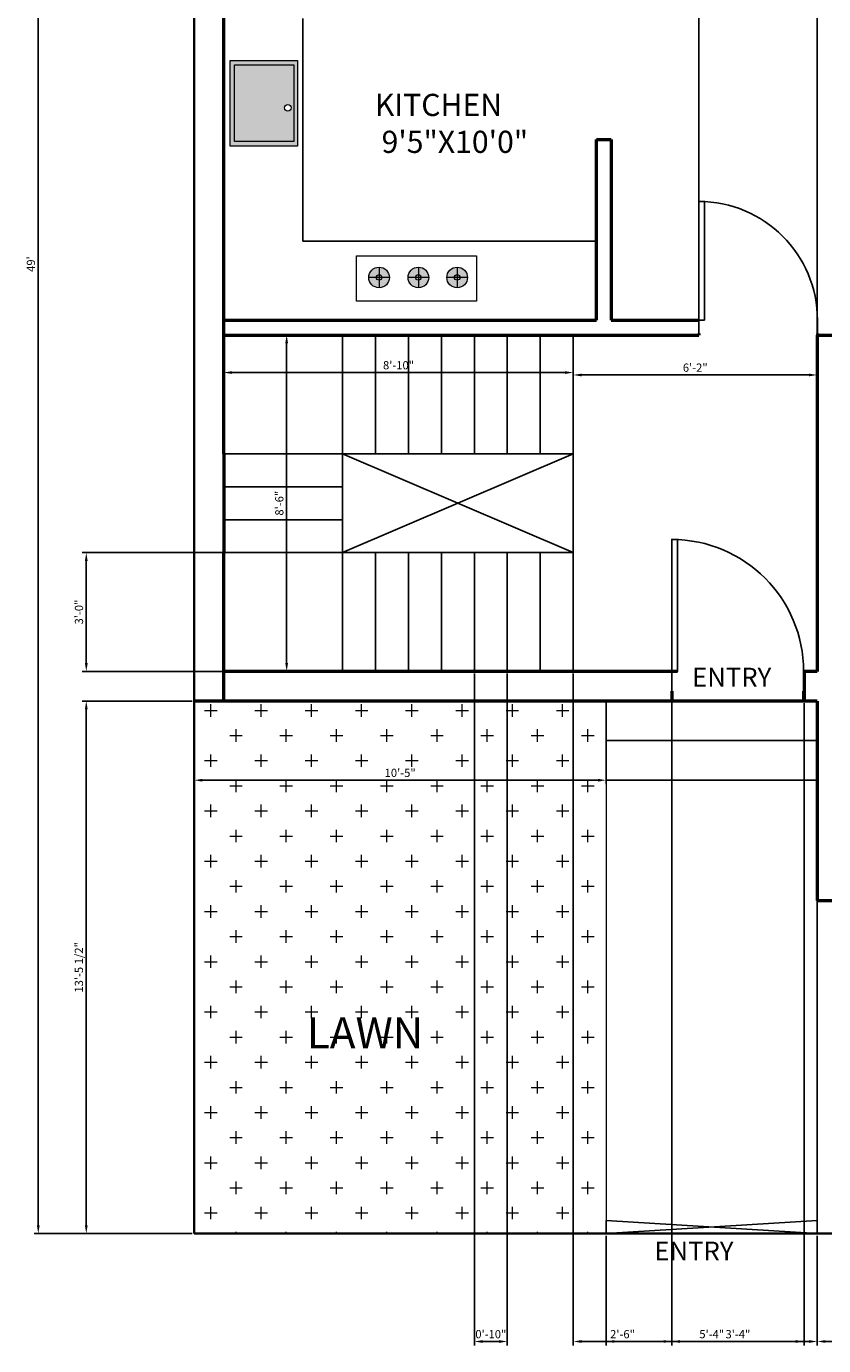
# Model space of a CAD drawing. Units: inches. Extents: x 1455 to 2044, y 1728 to 2439.
# Tile 1 of 4: x 1455 to 1697, y 1728 to 2128. Entities that reach past the tile are written whole.
import ezdxf

# ---------------------------------------------------------------- set-up
doc = ezdxf.new("R2010")
doc.units = ezdxf.units.IN
for name, color, linetype, lineweight in [('A-ANNO-DIMS', 2, 'Continuous', 18), ('A-ANNO-TEXT', 7, 'Continuous', 18), ('A-AREA-IDEN', 7, 'Continuous', 25), ('A-DOOR', 4, 'Continuous', 25), ('A-EQPM', 8, 'Continuous', 18), ('A-EQPM-PATT', 252, 'Continuous', 13), ('A-FLOR', 7, 'Continuous', 25), ('A-FLOR-CASE', 8, 'Continuous', 25), ('A-FLOR-FIXT', 9, 'Continuous', 18), ('A-FLOR-FIXT-PATT', 252, 'Continuous', 13), ('A-FLOR-STRS', 7, 'Continuous', 25), ('A-WALL', 7, 'Continuous', 50), ('C-PROP', 7, 'Continuous', 35), ('C-SITE-GATE', 1, 'Continuous', 25), ('L-PLNT', 3, 'Continuous', 18), ('L-PLNT-PATT', 3, 'Continuous', 13)]:
    doc.layers.add(name, color=color, linetype=linetype, lineweight=lineweight)
doc.styles.get("Standard").update_dxf_attribs({"font": 'arial.ttf'})
doc.dimstyles.new('ISO-25', dxfattribs={"dimtxt": 2.5, "dimasz": 2.5, "dimexe": 1.25, "dimexo": 0.625, "dimtad": 1, "dimlunit": 3, "dimtxsty": 'Standard', "dimcen": 2.5, "dimadec": 0, "dimazin": 0, "dimtfac": 1, "dimtmove": 0, "dimatfit": 3, "dimfxl": 1, "dimarcsym": 0})

# ---------------------------------------------------------------- blocks, each defined once
blk = doc.blocks.new('*D8')
at = {"layer": 'A-ANNO-DIMS', "color": 0, "lineweight": -2, "transparency": 16777216}
for p, q in [((1515.2, 2034.08), (1534.9, 2034.08)), ((1533.65, 2031.58), (1533.65, 1934.58)), ((1515.2, 1932.08), (1534.9, 1932.08))]:
    blk.add_line(p, q, dxfattribs=at)
at = {"layer": 'A-ANNO-DIMS', "color": 0, "transparency": 16777216}
for points in [[(1533.24, 2031.58), (1534.07, 2031.58), (1533.65, 2034.08)], [(1533.24, 1934.58), (1534.07, 1934.58), (1533.65, 1932.08)]]:
    blk.add_solid(points, dxfattribs=at)
at = {"layer": 'Defpoints', "color": 0, "transparency": 16777216}
for p in [(1514.58, 2034.08), (1514.58, 1932.08), (1533.65, 1932.08)]:
    blk.add_point(p, dxfattribs=at)
at = {"layer": 'A-ANNO-DIMS', "color": 0, "transparency": 16777216, "insert": (1531.75, 1983.08), "char_height": 2.5, "attachment_point": 5, "rotation": 90}
blk.add_mtext('8\'-6"', dxfattribs=at)
blk = doc.blocks.new('*D9')
at = {"layer": 'A-ANNO-DIMS', "color": 0, "lineweight": -2, "transparency": 16777216}
for p, q in [((1514.58, 2033.45), (1514.58, 2021.44)), ((1620.58, 2033.45), (1620.58, 2021.44)), ((1517.08, 2022.69), (1618.08, 2022.69))]:
    blk.add_line(p, q, dxfattribs=at)
at = {"layer": 'A-ANNO-DIMS', "color": 0, "transparency": 16777216}
for points in [[(1517.08, 2023.11), (1517.08, 2022.28), (1514.58, 2022.69)], [(1618.08, 2023.11), (1618.08, 2022.28), (1620.58, 2022.69)]]:
    blk.add_solid(points, dxfattribs=at)
at = {"layer": 'Defpoints', "color": 0, "transparency": 16777216}
for p in [(1514.58, 2034.08), (1620.58, 2034.08), (1620.58, 2022.69)]:
    blk.add_point(p, dxfattribs=at)
at = {"layer": 'A-ANNO-DIMS', "color": 0, "transparency": 16777216, "insert": (1567.58, 2024.59), "char_height": 2.5, "attachment_point": 5}
blk.add_mtext('8\'-10"', dxfattribs=at)
blk = doc.blocks.new('*D10')
at = {"layer": 'A-ANNO-DIMS', "color": 0, "lineweight": -2, "transparency": 16777216}
for p, q in [((1620.58, 2033.45), (1620.58, 2020.71)), ((1694.58, 2033.45), (1694.58, 2020.71)), ((1623.08, 2021.96), (1692.08, 2021.96))]:
    blk.add_line(p, q, dxfattribs=at)
at = {"layer": 'A-ANNO-DIMS', "color": 0, "transparency": 16777216}
for points in [[(1623.08, 2022.37), (1623.08, 2021.54), (1620.58, 2021.96)], [(1692.08, 2022.37), (1692.08, 2021.54), (1694.58, 2021.96)]]:
    blk.add_solid(points, dxfattribs=at)
at = {"layer": 'Defpoints', "color": 0, "transparency": 16777216}
for p in [(1620.58, 2034.08), (1694.58, 2034.08), (1694.58, 2021.96)]:
    blk.add_point(p, dxfattribs=at)
at = {"layer": 'A-ANNO-DIMS', "color": 0, "transparency": 16777216, "insert": (1657.58, 2023.86), "char_height": 2.5, "attachment_point": 5}
blk.add_mtext('6\'-2"', dxfattribs=at)
blk = doc.blocks.new('*U11')
for p, q in [((0, 0), (0, -6)), ((40, 0), (40, -6))]:
    blk.add_line(p, q)
blk.add_lwpolyline([(0, 0), (0, 40), (1.75, 40), (1.75, 0)], close=True)
blk.add_arc((0, 0), 40, 0, 90)
blk = doc.blocks.new('*U12')
for p, q in [((0, 0), (0, -4)), ((36, 0), (36, -4))]:
    blk.add_line(p, q)
blk.add_lwpolyline([(0, 0), (0, 36), (1.75, 36), (1.75, 0)], close=True)
blk.add_arc((0, 0), 36, 0, 90)
blk = doc.blocks.new('*D15')
at = {"layer": 'A-ANNO-DIMS', "color": 0, "lineweight": -2, "transparency": 16777216}
for p, q in [((1505.58, 1922.45), (1505.58, 1897.83)), ((1630.58, 1922.45), (1630.58, 1897.83)), ((1508.08, 1899.08), (1628.08, 1899.08))]:
    blk.add_line(p, q, dxfattribs=at)
at = {"layer": 'A-ANNO-DIMS', "color": 0, "transparency": 16777216}
for points in [[(1508.08, 1899.5), (1508.08, 1898.66), (1505.58, 1899.08)], [(1628.08, 1899.5), (1628.08, 1898.66), (1630.58, 1899.08)]]:
    blk.add_solid(points, dxfattribs=at)
at = {"layer": 'Defpoints', "color": 0, "transparency": 16777216}
for p in [(1505.58, 1923.08), (1630.58, 1923.08), (1630.58, 1899.08)]:
    blk.add_point(p, dxfattribs=at)
at = {"layer": 'A-ANNO-DIMS', "color": 0, "transparency": 16777216, "insert": (1568.08, 1900.98), "char_height": 2.5, "attachment_point": 5}
blk.add_mtext('10\'-5"', dxfattribs=at)
blk = doc.blocks.new('*D16')
at = {"layer": 'A-ANNO-DIMS', "color": 0, "lineweight": -2, "transparency": 16777216}
for p, q in [((1504.95, 2349.58), (1457.06, 2349.58)), ((1458.31, 2347.08), (1458.31, 1764.08)), ((1504.95, 1761.58), (1457.06, 1761.58))]:
    blk.add_line(p, q, dxfattribs=at)
at = {"layer": 'A-ANNO-DIMS', "color": 0, "transparency": 16777216}
for points in [[(1457.9, 2347.08), (1458.73, 2347.08), (1458.31, 2349.58)], [(1457.9, 1764.08), (1458.73, 1764.08), (1458.31, 1761.58)]]:
    blk.add_solid(points, dxfattribs=at)
at = {"layer": 'Defpoints', "color": 0, "transparency": 16777216}
for p in [(1505.58, 2349.58), (1458.31, 1761.58), (1505.58, 1761.58)]:
    blk.add_point(p, dxfattribs=at)
at = {"layer": 'A-ANNO-DIMS', "color": 0, "transparency": 16777216, "insert": (1456.41, 2055.58), "char_height": 2.5, "attachment_point": 5, "rotation": 90}
blk.add_mtext("49'", dxfattribs=at)
blk = doc.blocks.new('*D28')
at = {"layer": 'A-ANNO-DIMS', "color": 0, "lineweight": -2, "transparency": 16777216}
for p, q in [((1694.58, 1760.95), (1694.58, 1727.63)), ((1856.58, 1760.95), (1856.58, 1727.63)), ((1697.08, 1728.88), (1854.08, 1728.88))]:
    blk.add_line(p, q, dxfattribs=at)
at = {"layer": 'A-ANNO-DIMS', "color": 0, "transparency": 16777216}
for points in [[(1697.08, 1729.3), (1697.08, 1728.46), (1694.58, 1728.88)], [(1854.08, 1729.3), (1854.08, 1728.46), (1856.58, 1728.88)]]:
    blk.add_solid(points, dxfattribs=at)
at = {"layer": 'Defpoints', "color": 0, "transparency": 16777216}
for p in [(1694.58, 1761.58), (1856.58, 1761.58), (1856.58, 1728.88)]:
    blk.add_point(p, dxfattribs=at)
at = {"layer": 'A-ANNO-DIMS', "color": 0, "transparency": 16777216, "insert": (1775.58, 1730.78), "char_height": 2.5, "attachment_point": 5}
blk.add_mtext('13\'-6"', dxfattribs=at)
blk = doc.blocks.new('*D29')
at = {"layer": 'A-ANNO-DIMS', "color": 0, "lineweight": -2, "transparency": 16777216}
for p, q in [((1630.58, 1760.95), (1630.58, 1727.63)), ((1694.58, 1760.95), (1694.58, 1727.63)), ((1633.08, 1728.88), (1692.08, 1728.88))]:
    blk.add_line(p, q, dxfattribs=at)
at = {"layer": 'A-ANNO-DIMS', "color": 0, "transparency": 16777216}
for points in [[(1633.08, 1729.3), (1633.08, 1728.46), (1630.58, 1728.88)], [(1692.08, 1729.3), (1692.08, 1728.46), (1694.58, 1728.88)]]:
    blk.add_solid(points, dxfattribs=at)
at = {"layer": 'Defpoints', "color": 0, "transparency": 16777216}
for p in [(1630.58, 1761.58), (1694.58, 1761.58), (1694.58, 1728.88)]:
    blk.add_point(p, dxfattribs=at)
at = {"layer": 'A-ANNO-DIMS', "color": 0, "transparency": 16777216, "insert": (1662.58, 1730.78), "char_height": 2.5, "attachment_point": 5}
blk.add_mtext('5\'-4"', dxfattribs=at)
blk = doc.blocks.new('*D30')
at = {"layer": 'A-ANNO-DIMS', "color": 0, "lineweight": -2, "transparency": 16777216}
for p, q in [((1504.95, 1923.08), (1471.63, 1923.08)), ((1472.88, 1920.58), (1472.88, 1764.08)), ((1504.95, 1761.58), (1471.63, 1761.58))]:
    blk.add_line(p, q, dxfattribs=at)
at = {"layer": 'A-ANNO-DIMS', "color": 0, "transparency": 16777216}
for points in [[(1472.46, 1920.58), (1473.3, 1920.58), (1472.88, 1923.08)], [(1472.46, 1764.08), (1473.3, 1764.08), (1472.88, 1761.58)]]:
    blk.add_solid(points, dxfattribs=at)
at = {"layer": 'Defpoints', "color": 0, "transparency": 16777216}
for p in [(1505.58, 1923.08), (1472.88, 1761.58), (1505.58, 1761.58)]:
    blk.add_point(p, dxfattribs=at)
at = {"layer": 'A-ANNO-DIMS', "color": 0, "transparency": 16777216, "insert": (1470.96, 1842.33), "char_height": 2.5, "attachment_point": 5, "rotation": 90}
blk.add_mtext('13\'-5 1/2"', dxfattribs=at)
blk = doc.blocks.new('*D32')
at = {"layer": 'A-ANNO-DIMS', "color": 0, "lineweight": -2, "transparency": 16777216}
for p, q in [((1658.63, 2034.7), (1658.63, 2434.3)), ((1661.13, 2433.05), (1692.08, 2433.05)), ((1694.58, 2034.7), (1694.58, 2434.3))]:
    blk.add_line(p, q, dxfattribs=at)
at = {"layer": 'A-ANNO-DIMS', "color": 0, "transparency": 16777216}
for points in [[(1661.13, 2433.46), (1661.13, 2432.63), (1658.63, 2433.05)], [(1692.08, 2433.46), (1692.08, 2432.63), (1694.58, 2433.05)]]:
    blk.add_solid(points, dxfattribs=at)
at = {"layer": 'Defpoints', "color": 0, "transparency": 16777216}
for p in [(1694.58, 2433.05), (1658.63, 2034.08), (1694.58, 2034.08)]:
    blk.add_point(p, dxfattribs=at)
at = {"layer": 'A-ANNO-DIMS', "color": 0, "transparency": 16777216, "insert": (1676.61, 2434.95), "char_height": 2.5, "attachment_point": 5}
blk.add_mtext('3\'-0"', dxfattribs=at)
blk = doc.blocks.new('*D33')
at = {"layer": 'A-ANNO-DIMS', "color": 0, "lineweight": -2, "transparency": 16777216}
for p, q in [((1650.46, 1922.45), (1650.46, 1727.63)), ((1690.58, 1922.45), (1690.58, 1727.63)), ((1652.96, 1728.88), (1688.08, 1728.88))]:
    blk.add_line(p, q, dxfattribs=at)
at = {"layer": 'A-ANNO-DIMS', "color": 0, "transparency": 16777216}
for points in [[(1652.96, 1729.3), (1652.96, 1728.46), (1650.46, 1728.88)], [(1688.08, 1729.3), (1688.08, 1728.46), (1690.58, 1728.88)]]:
    blk.add_solid(points, dxfattribs=at)
at = {"layer": 'Defpoints', "color": 0, "transparency": 16777216}
for p in [(1650.46, 1923.08), (1690.58, 1923.08), (1690.58, 1728.88)]:
    blk.add_point(p, dxfattribs=at)
at = {"layer": 'A-ANNO-DIMS', "color": 0, "transparency": 16777216, "insert": (1670.52, 1730.78), "char_height": 2.5, "attachment_point": 5}
blk.add_mtext('3\'-4"', dxfattribs=at)
blk = doc.blocks.new('*D34')
at = {"layer": 'A-ANNO-DIMS', "color": 0, "lineweight": -2, "transparency": 16777216}
for p, q in [((1620.58, 1931.45), (1620.58, 1727.63)), ((1650.46, 1931.45), (1650.46, 1727.63)), ((1623.08, 1728.88), (1647.96, 1728.88))]:
    blk.add_line(p, q, dxfattribs=at)
at = {"layer": 'A-ANNO-DIMS', "color": 0, "transparency": 16777216}
for points in [[(1623.08, 1729.3), (1623.08, 1728.46), (1620.58, 1728.88)], [(1647.96, 1729.3), (1647.96, 1728.46), (1650.46, 1728.88)]]:
    blk.add_solid(points, dxfattribs=at)
at = {"layer": 'Defpoints', "color": 0, "transparency": 16777216}
for p in [(1620.58, 1932.08), (1650.46, 1932.07), (1650.46, 1728.88)]:
    blk.add_point(p, dxfattribs=at)
at = {"layer": 'A-ANNO-DIMS', "color": 0, "transparency": 16777216, "insert": (1635.52, 1730.78), "char_height": 2.5, "attachment_point": 5}
blk.add_mtext('2\'-6"', dxfattribs=at)
blk = doc.blocks.new('*D35')
at = {"layer": 'A-ANNO-DIMS', "color": 0, "lineweight": -2, "transparency": 16777216}
for p, q in [((1549.95, 1968.08), (1471.63, 1968.08)), ((1472.88, 1934.58), (1472.88, 1965.58)), ((1549.95, 1932.08), (1471.63, 1932.08))]:
    blk.add_line(p, q, dxfattribs=at)
at = {"layer": 'A-ANNO-DIMS', "color": 0, "transparency": 16777216}
for points in [[(1472.46, 1965.58), (1473.3, 1965.58), (1472.88, 1968.08)], [(1472.46, 1934.58), (1473.3, 1934.58), (1472.88, 1932.08)]]:
    blk.add_solid(points, dxfattribs=at)
at = {"layer": 'Defpoints', "color": 0, "transparency": 16777216}
for p in [(1472.88, 1968.08), (1550.58, 1968.08), (1550.58, 1932.08)]:
    blk.add_point(p, dxfattribs=at)
at = {"layer": 'A-ANNO-DIMS', "color": 0, "transparency": 16777216, "insert": (1470.98, 1950.08), "char_height": 2.5, "attachment_point": 5, "rotation": 90}
blk.add_mtext('3\'-0"', dxfattribs=at)
blk = doc.blocks.new('*D36')
at = {"layer": 'A-ANNO-DIMS', "color": 0, "lineweight": -2, "transparency": 16777216}
for p, q in [((1590.58, 1931.45), (1590.58, 1727.63)), ((1600.58, 1931.45), (1600.58, 1727.63)), ((1593.08, 1728.88), (1598.08, 1728.88))]:
    blk.add_line(p, q, dxfattribs=at)
at = {"layer": 'A-ANNO-DIMS', "color": 0, "transparency": 16777216}
for points in [[(1593.08, 1729.3), (1593.08, 1728.46), (1590.58, 1728.88)], [(1598.08, 1729.3), (1598.08, 1728.46), (1600.58, 1728.88)]]:
    blk.add_solid(points, dxfattribs=at)
at = {"layer": 'Defpoints', "color": 0, "transparency": 16777216}
for p in [(1590.58, 1932.08), (1600.58, 1932.08), (1600.58, 1728.88)]:
    blk.add_point(p, dxfattribs=at)
at = {"layer": 'A-ANNO-DIMS', "color": 0, "transparency": 16777216, "insert": (1595.58, 1730.78), "char_height": 2.5, "attachment_point": 5}
blk.add_mtext('0\'-10"', dxfattribs=at)

msp = doc.modelspace()

# ---------------------------------------------------------------- hatches: boundary and pattern name
at = {"layer": 'A-EQPM-PATT'}
h = msp.add_hatch(color=256, dxfattribs=at)
h.dxf.hatch_style = 1
h.paths.add_polyline_path([(1561.682, 2054.661), (1561.682, 2052.357, -0.4142136), (1562.508, 2051.532), (1564.812, 2051.532, 0.4142136)])
h.paths.add_polyline_path([(1561.682, 2052.357), (1561.682, 2054.661, 0.4142136), (1558.553, 2051.532), (1560.857, 2051.532, -0.4142136)])
h.paths.add_polyline_path([(1561.682, 2050.706, -0.4142136), (1560.857, 2051.532), (1558.553, 2051.532, 0.4142136), (1561.682, 2048.402)])
h.paths.add_polyline_path([(1564.812, 2051.532), (1562.508, 2051.532, -0.4142136), (1561.682, 2050.706), (1561.682, 2048.402, 0.4142136)])
h.paths.add_polyline_path([(1573.604, 2054.661), (1573.604, 2052.357, -0.4142136), (1574.43, 2051.532), (1576.734, 2051.532, 0.4142136)])
h.paths.add_polyline_path([(1573.604, 2052.357), (1573.604, 2054.661, 0.4142136), (1570.474, 2051.532), (1572.779, 2051.532, -0.4142136)])
h.paths.add_polyline_path([(1573.604, 2050.706, -0.4142136), (1572.779, 2051.532), (1570.474, 2051.532, 0.4142136), (1573.604, 2048.402)])
h.paths.add_polyline_path([(1576.734, 2051.532), (1574.43, 2051.532, -0.4142136), (1573.604, 2050.706), (1573.604, 2048.402, 0.4142136)])
h.paths.add_polyline_path([(1585.367, 2054.661), (1585.367, 2052.357, -0.4142136), (1586.192, 2051.532), (1588.496, 2051.532, 0.4142136)])
h.paths.add_polyline_path([(1588.496, 2051.532), (1586.192, 2051.532, -0.4142136), (1585.367, 2050.706), (1585.367, 2048.402, 0.4142136)])
h.paths.add_polyline_path([(1585.367, 2050.706, -0.4142136), (1584.541, 2051.532), (1582.237, 2051.532, 0.4142136), (1585.367, 2048.402)])
h.paths.add_polyline_path([(1585.367, 2054.661, 0.4142136), (1582.237, 2051.532), (1584.541, 2051.532, -0.4142136), (1585.367, 2052.357)])
h = msp.add_hatch(color=256, dxfattribs=at)
h.dxf.hatch_style = 1
h.paths.add_polyline_path([(1561.682, 2052.357, 0.4142136), (1560.857, 2051.532), (1561.682, 2051.532)])
h.paths.add_polyline_path([(1561.682, 2052.357), (1561.682, 2051.532), (1562.508, 2051.532, 0.4142136)])
h.paths.add_polyline_path([(1562.508, 2051.532), (1561.682, 2051.532), (1561.682, 2050.706, 0.4142136)])
h.paths.add_polyline_path([(1561.682, 2051.532), (1560.857, 2051.532, 0.4142136), (1561.682, 2050.706)])
h.paths.add_polyline_path([(1574.43, 2051.532), (1573.604, 2051.532), (1573.604, 2050.706, 0.4142136)])
h.paths.add_polyline_path([(1573.604, 2052.357), (1573.604, 2051.532), (1574.43, 2051.532, 0.4142136)])
h.paths.add_polyline_path([(1573.604, 2052.357, 0.4142136), (1572.779, 2051.532), (1573.604, 2051.532)])
h.paths.add_polyline_path([(1573.604, 2051.532), (1572.779, 2051.532, 0.4142136), (1573.604, 2050.706)])
h.paths.add_polyline_path([(1585.367, 2052.357, 0.4142136), (1584.541, 2051.532), (1585.367, 2051.532)])
h.paths.add_polyline_path([(1585.367, 2052.357), (1585.367, 2051.532), (1586.192, 2051.532, 0.4142136)])
h.paths.add_polyline_path([(1586.192, 2051.532), (1585.367, 2051.532), (1585.367, 2050.706, 0.4142136)])
h.paths.add_polyline_path([(1585.367, 2051.532), (1584.541, 2051.532, 0.4142136), (1585.367, 2050.706)])
at = {"layer": 'A-FLOR-FIXT-PATT'}
h = msp.add_hatch(color=256, dxfattribs=at)
h.dxf.hatch_style = 1
h.paths.add_polyline_path([(1536.984, 2117.369), (1516.561, 2117.369), (1516.561, 2091.312), (1536.984, 2091.312)])
h.paths.add_polyline_path([(1535.842, 2115.995), (1535.842, 2092.725), (1517.855, 2092.725), (1517.855, 2115.995)], flags=16)
h.paths.add_polyline_path([(1534.977, 2102.979, -1), (1532.975, 2102.979, -1)], flags=0)
h = msp.add_hatch(color=256, dxfattribs=at)
h.dxf.hatch_style = 1
h.paths.add_polyline_path([(1535.842, 2115.995), (1517.855, 2115.995), (1517.855, 2092.725), (1535.842, 2092.725)])
h.paths.add_polyline_path([(1534.977, 2102.979, -1), (1532.975, 2102.979, -1)], flags=16)
at = {"layer": 'L-PLNT-PATT'}
h = msp.add_hatch(dxfattribs=at)
h.set_pattern_fill('CROSS', color=256, scale=1.2)
h.paths.add_polyline_path([(1505.58, 1923.079), (1505.58, 1761.579), (1630.58, 1761.579), (1630.58, 1923.079)])
h.paths.add_polyline_path([(1562.898, 1898.382), (1573.045, 1898.382), (1573.045, 1903.533), (1562.898, 1903.533)], flags=24)

# ---------------------------------------------------------------- linework, layer by layer
at = {"layer": 'A-EQPM'}
for p, q in [((1561.682, 2054.661), (1561.682, 2048.402)), ((1573.604, 2054.661), (1573.604, 2048.402)), ((1585.367, 2054.661), (1585.367, 2048.402)), ((1564.812, 2051.532), (1558.553, 2051.532)), ((1576.734, 2051.532), (1570.474, 2051.532)), ((1588.496, 2051.532), (1582.237, 2051.532))]:
    msp.add_line(p, q, dxfattribs=at)
msp.add_lwpolyline([(1554.842, 2058.043), (1591.244, 2058.043), (1591.244, 2044.351), (1554.842, 2044.351)], close=True, dxfattribs=at)
for centre, radius in [((1561.682, 2051.532), 3.13), ((1561.682, 2051.532), 0.826), ((1573.604, 2051.532), 3.13), ((1573.604, 2051.532), 0.826), ((1585.367, 2051.532), 3.13), ((1585.367, 2051.532), 0.826)]:
    msp.add_circle(centre, radius, dxfattribs=at)
at = {"layer": 'A-FLOR'}
msp.add_line((1694.58, 1862.579), (1694.58, 1761.579), dxfattribs=at)
at = {"layer": 'A-FLOR-CASE'}
for p, q in [((1514.58, 2130.055), (1514.58, 2038.579)), ((1538.58, 2130.055), (1538.58, 2062.579)), ((1538.58, 2062.579), (1627.58, 2062.579))]:
    msp.add_line(p, q, dxfattribs=at)
at = {"layer": 'A-FLOR-FIXT'}
for points in [[(1516.561, 2117.369), (1536.984, 2117.369), (1536.984, 2091.312), (1516.561, 2091.312)], [(1517.855, 2115.995), (1535.842, 2115.995), (1535.842, 2092.725), (1517.855, 2092.725)]]:
    msp.add_lwpolyline(points, close=True, dxfattribs=at)
msp.add_circle((1533.976, 2102.979), 1.001, dxfattribs=at)
at = {"layer": 'A-FLOR-STRS'}
for p, q in [((1514.58, 2034.079), (1620.58, 2034.079)), ((1550.58, 2034.079), (1550.58, 1998.079)), ((1560.58, 2034.079), (1560.58, 1998.079)), ((1570.58, 2034.079), (1570.58, 1998.079)), ((1580.58, 2034.079), (1580.58, 1998.079)), ((1590.58, 2034.079), (1590.58, 1998.079)), ((1600.58, 2034.079), (1600.58, 1998.079)), ((1610.58, 2034.079), (1610.58, 1998.079)), ((1620.58, 2034.079), (1620.58, 1932.079)), ((1620.58, 2034.079), (1620.58, 1998.079)), ((1620.58, 1998.079), (1514.58, 1998.079)), ((1620.58, 1998.079), (1550.58, 1968.079)), ((1550.58, 1998.079), (1620.58, 1968.079)), ((1550.58, 1998.079), (1550.58, 1968.079)), ((1514.58, 1988.079), (1550.58, 1988.079)), ((1550.58, 1978.079), (1514.58, 1978.079)), ((1620.58, 1968.079), (1514.58, 1968.079)), ((1550.58, 1932.079), (1550.58, 1968.079)), ((1560.58, 1932.079), (1560.58, 1968.079)), ((1570.58, 1932.079), (1570.58, 1968.079)), ((1580.58, 1932.079), (1580.58, 1968.079)), ((1590.58, 1932.079), (1590.58, 1968.079)), ((1600.58, 1932.079), (1600.58, 1968.079)), ((1610.58, 1932.079), (1610.58, 1968.079)), ((1620.58, 1932.079), (1620.58, 1968.079)), ((1630.58, 1923.079), (1630.58, 1911.079)), ((1630.58, 1911.079), (1694.58, 1911.079)), ((1630.58, 1899.079), (1694.58, 1899.079))]:
    msp.add_line(p, q, dxfattribs=at)
at = {"layer": 'A-WALL'}
for p, q in [((1514.58, 1998.079), (1514.58, 2340.579)), ((1627.58, 2062.579), (1627.58, 2093.34)), ((1627.58, 2093.34), (1632.08, 2093.34)), ((1632.08, 2093.34), (1632.08, 2038.579)), ((1627.58, 2038.579), (1627.58, 2062.579)), ((1514.58, 2038.579), (1627.58, 2038.579)), ((1632.08, 2038.579), (1651.58, 2038.579)), ((1651.58, 2038.579), (1658.632, 2038.579)), ((1514.58, 2034.079), (1651.58, 2034.079)), ((1620.58, 2034.079), (1658.632, 2034.079)), ((1658.632, 2034.583), (1658.632, 2034.079)), ((1694.58, 2034.079), (1694.58, 1932.079)), ((1694.58, 2034.079), (1699.08, 2034.079)), ((1694.632, 2034.583), (1694.632, 2034.079)), ((1514.58, 1998.079), (1514.58, 1968.079)), ((1514.58, 1923.079), (1514.58, 1968.079)), ((1694.58, 1932.079), (1690.58, 1932.079)), ((1690.58, 1932.079), (1690.58, 1923.079)), ((1650.459, 1926.074), (1650.459, 1923.079)), ((1690.459, 1926.074), (1690.459, 1923.079)), ((1514.58, 1923.079), (1505.58, 1923.079)), ((1694.58, 1923.079), (1694.58, 1862.579))]:
    msp.add_line(p, q, dxfattribs=at)
for points in [[(1652.209, 1932.079), (1620.58, 1932.079), (1514.58, 1932.079)], [(1694.58, 1932.079), (1690.459, 1932.079)], [(1694.58, 1923.079), (1620.58, 1923.079), (1514.58, 1923.079)], [(1694.58, 1862.579), (1705.504, 1862.579)]]:
    msp.add_lwpolyline(points, dxfattribs=at)
at = {"layer": 'C-PROP'}
for p, q in [((1505.58, 1761.579), (1505.58, 2349.579)), ((1856.58, 1761.579), (1505.58, 1761.579))]:
    msp.add_line(p, q, dxfattribs=at)
at = {"layer": 'C-SITE-GATE'}
for p, q in [((1630.58, 1761.579), (1630.58, 1765.579)), ((1694.58, 1761.579), (1630.58, 1765.579)), ((1694.58, 1765.579), (1630.58, 1761.579)), ((1694.58, 1765.579), (1694.58, 1761.579))]:
    msp.add_line(p, q, dxfattribs=at)
at = {"layer": 'L-PLNT'}
for p, q in [((1505.58, 1923.079), (1630.58, 1923.079)), ((1630.58, 1923.079), (1630.58, 1761.579))]:
    msp.add_line(p, q, dxfattribs=at)

# ---------------------------------------------------------------- block references
at = {"layer": 'A-DOOR'}
for name, p in [('*U12', (1658.632, 2038.583)), ('*U11', (1650.459, 1932.074))]:
    msp.add_blockref(name, p, dxfattribs=at)

# ---------------------------------------------------------------- texts
at = {"layer": 'A-ANNO-TEXT', "char_height": 5.7222, "attachment_point": 1}
for insert in [(1656.616, 1933.189), (1645.165, 1759.166)]:
    msp.add_mtext_dynamic_manual_height_columns('ENTRY', width=92.73423, gutter_width=28.611, heights=[0], dxfattribs=dict(at, insert=insert))
at = {"layer": 'A-AREA-IDEN', "attachment_point": 1}
for s, width, gutter_width, insert, char_height in [('KITCHEN\\P 9\'5"X10\'0"', 99.14603, 33.578, (1560.385, 2107.211), 6.71568), ('LAWN', 268.14673, 47.069, (1539.76, 1827.179), 9.4138)]:
    msp.add_mtext_dynamic_manual_height_columns(s, width=width, gutter_width=gutter_width, heights=[0], dxfattribs=dict(at, insert=insert, char_height=char_height))

# ---------------------------------------------------------------- dimensions: what is measured, and where the dimension line sits
at = {"layer": 'A-ANNO-DIMS'}
for base, p1, p2, override, picture, middle in [((1694.58, 2433.046), (1658.632, 2034.079), (1694.58, 2034.079), {"dimdec": 1, "dimlfac": 1, "dimrnd": 0, "dimzin": 1, "dimdsep": 46, "dimlunit": 4, "dimfrac": 2}, '*D32', (1676.606, 2434.948)), ((1620.58, 2022.692), (1514.58, 2034.079), (1620.58, 2034.079), {"dimclrd": 0, "dimclre": 0, "dimclrt": 0}, '*D9', (1567.58, 2024.594)), ((1694.58, 2021.957), (1620.58, 2034.079), (1694.58, 2034.079), {"dimclrd": 0, "dimclre": 0, "dimclrt": 0}, '*D10', (1657.58, 2023.858)), ((1600.58, 1728.879), (1590.58, 1932.079), (1600.58, 1932.079), {"dimdec": 1, "dimlfac": 1, "dimrnd": 0, "dimzin": 1, "dimdsep": 46, "dimlunit": 4, "dimfrac": 2}, '*D36', (1595.58, 1730.78)), ((1650.459, 1728.879), (1620.58, 1932.079), (1650.459, 1932.074), {"dimdec": 1, "dimlfac": 1, "dimrnd": 0, "dimzin": 1, "dimdsep": 46, "dimlunit": 4, "dimfrac": 2}, '*D34', (1635.519, 1730.78)), ((1630.58, 1899.079), (1505.58, 1923.079), (1630.58, 1923.079), {"dimclrd": 0, "dimclre": 0, "dimclrt": 0}, '*D15', (1568.08, 1900.98)), ((1690.58, 1728.879), (1650.459, 1923.079), (1690.58, 1923.079), {"dimdec": 1, "dimlfac": 1, "dimrnd": 0, "dimzin": 1, "dimdsep": 46, "dimlunit": 4, "dimfrac": 2}, '*D33', (1670.519, 1730.781)), ((1694.58, 1728.879), (1630.58, 1761.579), (1694.58, 1761.579), {"dimdec": 1, "dimlfac": 1, "dimrnd": 0, "dimzin": 1, "dimdsep": 46, "dimlunit": 4, "dimfrac": 2}, '*D29', (1662.58, 1730.775)), ((1856.58, 1728.879), (1694.58, 1761.579), (1856.58, 1761.579), {"dimdec": 1, "dimlfac": 1, "dimrnd": 0, "dimzin": 1, "dimdsep": 46, "dimlunit": 4, "dimfrac": 2}, '*D28', (1775.58, 1730.781))]:
    dim = msp.add_linear_dim(base=base, p1=p1, p2=p2, dimstyle='ISO-25', override=override, dxfattribs=at)
    dim.commit()
    dim.dimension.update_dxf_attribs({"geometry": picture, "text_midpoint": middle})
for base, p1, p2, override, picture, middle in [((1458.313, 1761.579), (1505.58, 2349.579), (1505.58, 1761.579), {"dimclrd": 0, "dimclre": 0, "dimclrt": 0}, '*D16', (1456.412, 2055.579)), ((1533.653, 1932.079), (1514.58, 2034.079), (1514.58, 1932.079), {"dimclrd": 0, "dimclre": 0, "dimclrt": 0}, '*D8', (1531.751, 1983.079)), ((1472.88, 1968.079), (1550.58, 1932.079), (1550.58, 1968.079), {"dimdec": 1, "dimlfac": 1, "dimrnd": 0, "dimzin": 1, "dimdsep": 46, "dimlunit": 4, "dimfrac": 2}, '*D35', (1470.977, 1950.079)), ((1472.88, 1761.579), (1505.58, 1923.079), (1505.58, 1761.579), {"dimdec": 1, "dimlfac": 1, "dimrnd": 0, "dimzin": 1, "dimdsep": 46, "dimlunit": 4, "dimfrac": 2}, '*D30', (1470.961, 1842.329))]:
    dim = msp.add_linear_dim(base=base, p1=p1, p2=p2, angle=90, dimstyle='ISO-25', override=override, dxfattribs=at)
    dim.commit()
    dim.dimension.update_dxf_attribs({"geometry": picture, "text_midpoint": middle})

doc.saveas('drawing.dxf')
